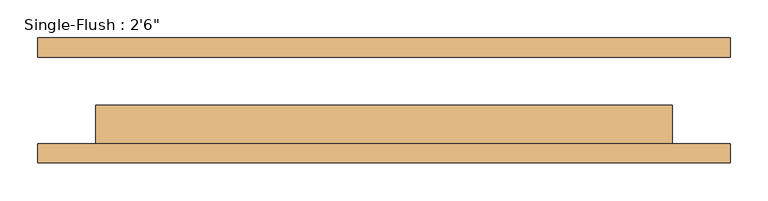
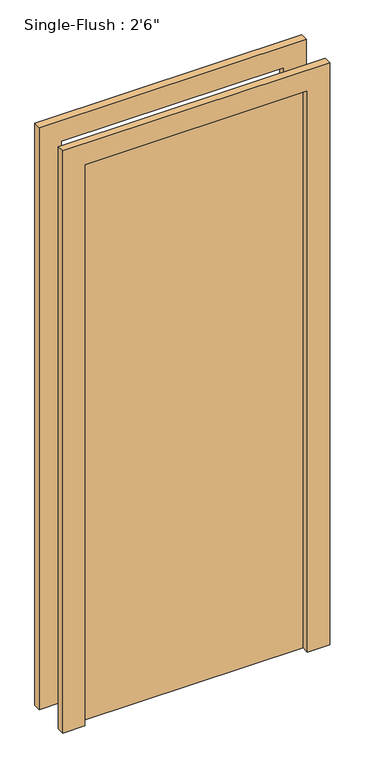
"""IFC4 building model written with IfcOpenShell, lengths in millimetres: door geometry."""

from ifc_helpers import new_model, si_unit, frame, origin, origin_with_axes, place, context, project, spatial, polyline, outline, extrude, source, transform, mapped, element, save


def door_f2b275c1(model_context):
    return source(origin(), model_context, "Body", "SweptSolid", [
        extrude(outline(polyline([(2108.2, -457.2), (0.0, -457.2), (0.0, -381.0), (2032.0, -381.0), (2032.0, 381.0), (0.0, 381.0), (0.0, 457.2), (2108.2, 457.2), (2108.2, -457.2)])), frame((0.0, -82.55, 0.0), z_axis=(0.0, 1.0, 0.0), x_axis=(0.0, 0.0, 1.0)), (0.0, 0.0, 1.0), 25.4),
        extrude(outline(polyline([(2108.2, 457.2), (2108.2, -457.2), (0.0, -457.2), (0.0, -381.0), (2032.0, -381.0), (2032.0, 381.0), (0.0, 381.0), (0.0, 457.2), (2108.2, 457.2)])), frame((0.0, 57.15, 0.0), z_axis=(0.0, 1.0, 0.0), x_axis=(0.0, 0.0, 1.0)), (0.0, 0.0, 1.0), 25.4),
        extrude(outline(polyline([(381.0, -6.35), (381.0, -57.15), (-381.0, -57.15), (-381.0, -6.35), (381.0, -6.35)])), origin_with_axes(), (0.0, 0.0, 1.0), 2032.0),
    ])


if __name__ == "__main__":
    model = new_model("IFC4")
    model_context = context("Model", 3, world=origin())
    ifc_project = project(units=[si_unit("LENGTHUNIT", "METRE", prefix="MILLI")], contexts=[model_context])
    site = spatial("IfcSite", under=ifc_project)
    building = spatial("IfcBuilding", under=site)
    placement = place(None, origin())
    door_shape = door_f2b275c1(model_context)
    element("IfcDoor", 1, ObjectType="Single-Flush : 2'6\"", at=placement, inside=building, context=model_context, shape_type="MappedRepresentation", body=[
        mapped(door_shape, transform((0.0, 0.0, 0.0), x_axis=(1.0, 0.0, 0.0), y_axis=(0.0, 1.0, 0.0), z_axis=(0.0, 0.0, 1.0))),
    ])
    save(model, "model.ifc")

# Revit data of these elements
# Type "Single-Flush : 2'6\""
#   Type Mark = "9"
#   Construction Type Id = "MDOOR"
#   Assembly Code = "C1020"
#   Analytic Construction = "Metal"
#   Thickness = 0' - 2"
#   Heat Transfer Coefficient (U) = 0.651978 BTU/(h·ft²·°F)
#   Height = 6' - 8"
#   Trim Projection Ext = 0' - 1"
#   Trim Projection Int = 0' - 1"
#   Trim Width = 0' - 3"
#   Width = 2' - 6"
#   Define Thermal Properties by = 1
#   Door Material = Door - Panel
#   Frame Material = Door - Frame
#   Visual Light Transmittance = 0
#   Solar Heat Gain Coefficient = 0
#   Function = (empty or 0)
#   Wall Closure = (empty or 0)
# Element 1 (IfcDoor, "Single-Flush : 2'6\"")
#   Materials on its faces: "Door - Frame", "Door - Panel"
# Materials
#   "Door - Panel": class "Wood", colour RGB 210 159 95, transparency 0, Cost = 0
#   "Door - Frame": colour RGB 118 70 51, transparency 0, Cost = 0
